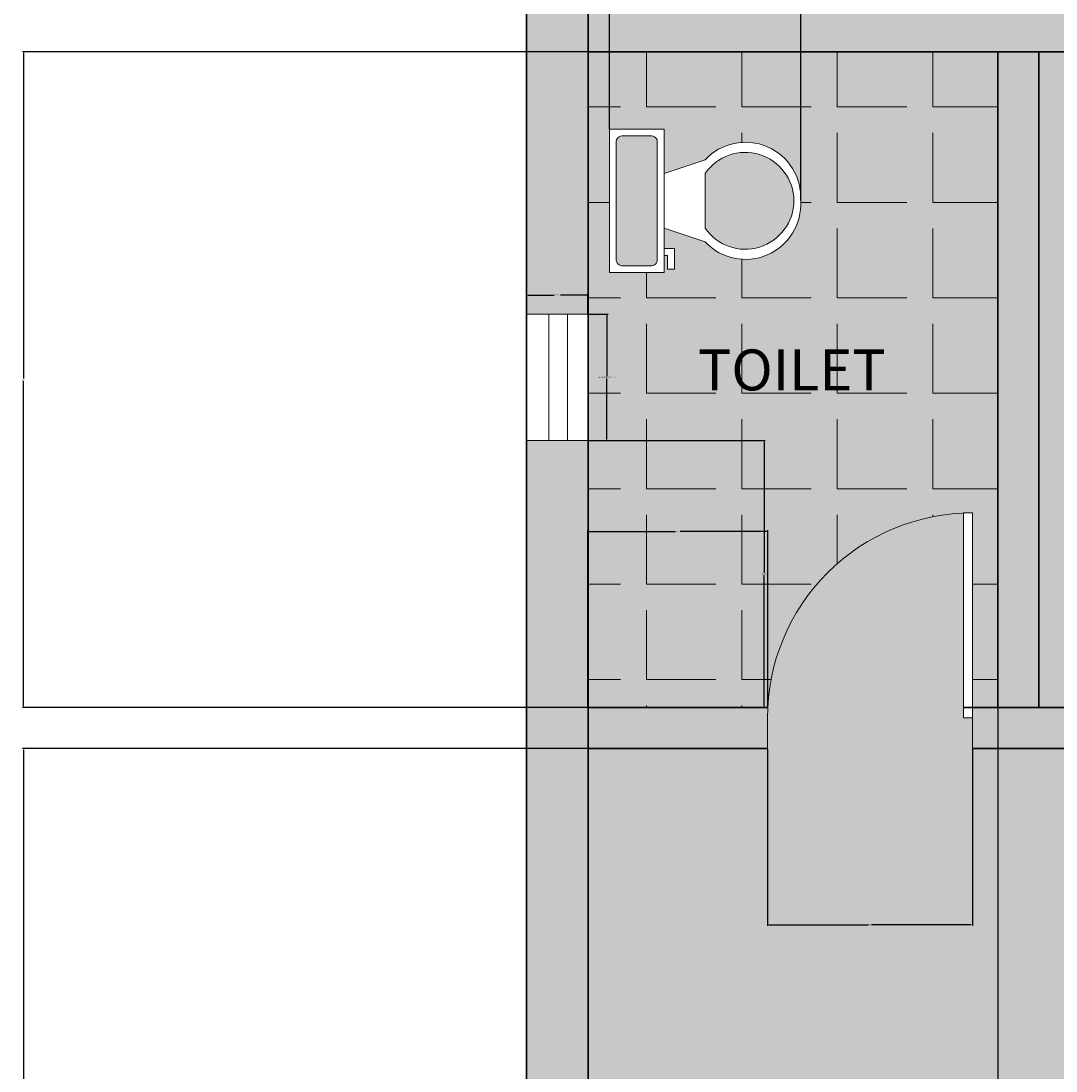
# Model space of a CAD drawing. Units: inches. Extents: x 3024 to 3952, y 1308 to 1863.
# Tile 2 of 29: x 3024 to 3175, y 1479 to 1633. Entities that reach past the tile are written whole.
import ezdxf

# ---------------------------------------------------------------- set-up
doc = ezdxf.new("R2010")
doc.units = ezdxf.units.IN
for name, color, linetype, lineweight in [('A-ANNO-DIMS', 2, 'Continuous', 18), ('A-AREA-IDEN', 7, 'Continuous', 18), ('A-DOOR', 4, 'Continuous', 18), ('A-FLOR-FIXT', 9, 'Continuous', 18), ('A-FLOR-FIXT-PATT', 7, 'Continuous', 13), ('A-FLOR-TILE-PATT', 7, 'Continuous', 13), ('A-GLAZ', 4, 'Continuous', 18), ('A-WALL', 7, 'Continuous', 35)]:
    doc.layers.add(name, color=color, linetype=linetype, lineweight=lineweight)
doc.layers.add('A-FLOR-PATT', color=254, linetype='Continuous', lineweight=13, true_color=0xfeeab9)
doc.layers.add('A-WALL-PATT', color=254, linetype='Continuous', lineweight=13, true_color=0xcecce6)
doc.styles.get("Standard").update_dxf_attribs({"font": 'arial.ttf'})
doc.dimstyles.get("Standard").update_dxf_attribs({"dimtxt": 0.18, "dimasz": 0.18, "dimexe": 0.18, "dimexo": 0.0625, "dimgap": 0.09, "dimtad": 0, "dimtih": 1, "dimtoh": 1, "dimdec": 4, "dimzin": 0, "dimdsep": 46, "dimtxsty": 'Standard', "dimcen": 0.09, "dimadec": 0, "dimazin": 0, "dimtfac": 1, "dimtdec": 4, "dimtofl": 0, "dimtmove": 0, "dimatfit": 3, "dimfxl": 1, "dimtolj": 1, "dimtzin": 0, "dimarcsym": 0})

# ---------------------------------------------------------------- blocks, each defined once
blk = doc.blocks.new('*U10')
for p, q in [((0, 0), (0, 6)), ((40, 0), (40, 6))]:
    blk.add_line(p, q)
blk.add_lwpolyline([(0, 0), (0, -40), (1.75, -40), (1.75, 0)], close=True)
blk.add_arc((0, 0), 40, 270, 0)
blk = doc.blocks.new('*U12')
for p, q in [((9.5, -6), (9.5, -2)), ((-10, -8.5), (-8, -8.5)), ((-10, -9.5), (-10, -8.5)), ((-8, -8.5), (-8, -8)), ((-7, -8), (-7, -9.5)), ((-4, -8), (-6, -14)), ((4, -8), (6, -14)), ((-7, -9.5), (-10, -9.5)), ((4, -14), (-4, -14))]:
    blk.add_line(p, q)
blk.add_lwpolyline([(10.5, -8), (10.5, 0), (-10.5, 0), (-10.5, -8)], close=True)
for points in [[(8.5, -1), (-8.5, -1)], [(-9.5, -2), (-9.5, -6)], [(-8.5, -7), (8.5, -7)]]:
    blk.add_lwpolyline(points)
for centre, radius, start, end in [((-8.625, -1.875), 0.8839, 81.8699, 188.1301), ((8.625, -1.875), 0.8839, 351.8699, 98.1301), ((-8.625, -6.125), 0.8839, 171.869898, 278.1301), ((8.625, -6.125), 0.8839, 261.8699, 8.1301), ((-0.4772, -19.9188), 8.0953, 133.01722, 273.38), ((0.0374, -19.8731), 7.127, 124.50543, 269.7), ((-0.0373, -19.8731), 7.127, 270.3, 55.4946), ((0.4773, -19.9188), 8.0953, 266.62, 46.9828)]:
    blk.add_arc(centre, radius, start, end)
blk = doc.blocks.new('WIN-BATH-18p5IN')
for p, q in [((0, 5.99), (0, 9)), ((18.52, 6.41), (18.52, 9)), ((18.52, 6.41), (18.52, 5.99)), ((0, 3.28), (0, 0)), ((18.52, 3.69), (18.52, 0))]:
    blk.add_line(p, q)
blk.add_lwpolyline([(0, 5.99), (18.52, 5.99), (18.52, 3.28), (0, 3.28)], close=True)
blk = doc.blocks.new('*D26')
at = {"layer": 'A-ANNO-DIMS', "color": 0, "lineweight": -2, "transparency": 16777216}
for p, q in [((3106.83, 1590.21), (3109.72, 1590.21)), ((3109.54, 1590.03), (3109.54, 1581.14)), ((3109.54, 1571.87), (3109.54, 1580.77)), ((3106.83, 1571.69), (3109.72, 1571.69))]:
    blk.add_line(p, q, dxfattribs=at)
at = {"layer": 'A-ANNO-DIMS', "color": 0, "transparency": 16777216}
for points in [[(3109.51, 1590.03), (3109.57, 1590.03), (3109.54, 1590.21)], [(3109.51, 1571.87), (3109.57, 1571.87), (3109.54, 1571.69)]]:
    blk.add_solid(points, dxfattribs=at)
at = {"layer": 'Defpoints', "color": 0, "transparency": 16777216}
for p in [(3106.76, 1590.21), (3106.76, 1571.69), (3109.54, 1571.69)]:
    blk.add_point(p, dxfattribs=at)
at = {"layer": 'A-ANNO-DIMS', "color": 0, "transparency": 16777216, "insert": (3109.54, 1580.95), "char_height": 0.18, "attachment_point": 5}
blk.add_mtext('\\A1;BATH WINDOW 19 TYP.', dxfattribs=at)
blk = doc.blocks.new('*D27')
at = {"layer": 'A-ANNO-DIMS', "color": 0, "lineweight": -2, "transparency": 16777216}
for p, q in [((3097.76, 1590.28), (3097.76, 1593.17)), ((3097.94, 1592.99), (3101.81, 1592.99)), ((3106.58, 1592.99), (3102.72, 1592.99)), ((3106.76, 1590.28), (3106.76, 1593.17))]:
    blk.add_line(p, q, dxfattribs=at)
at = {"layer": 'A-ANNO-DIMS', "color": 0, "transparency": 16777216}
for points in [[(3097.94, 1593.02), (3097.94, 1592.96), (3097.76, 1592.99)], [(3106.58, 1593.02), (3106.58, 1592.96), (3106.76, 1592.99)]]:
    blk.add_solid(points, dxfattribs=at)
at = {"layer": 'Defpoints', "color": 0, "transparency": 16777216}
for p in [(3106.76, 1592.99), (3097.76, 1590.21), (3106.76, 1590.21)]:
    blk.add_point(p, dxfattribs=at)
at = {"layer": 'A-ANNO-DIMS', "color": 0, "transparency": 16777216, "insert": (3102.26, 1592.99), "char_height": 0.18, "attachment_point": 5}
blk.add_mtext('\\A1;9 TYP.', dxfattribs=at)
blk = doc.blocks.new('*D43')
at = {"layer": 'A-ANNO-DIMS', "color": 0, "lineweight": -2, "transparency": 16777216}
for p, q in [((3106.7, 1628.61), (3023.95, 1628.61)), ((3024.13, 1628.43), (3024.13, 1580.79)), ((3024.13, 1532.79), (3024.13, 1580.42)), ((3106.7, 1532.61), (3023.95, 1532.61))]:
    blk.add_line(p, q, dxfattribs=at)
at = {"layer": 'A-ANNO-DIMS', "color": 0, "transparency": 16777216}
for points in [[(3024.1, 1628.43), (3024.16, 1628.43), (3024.13, 1628.61)], [(3024.1, 1532.79), (3024.16, 1532.79), (3024.13, 1532.61)]]:
    blk.add_solid(points, dxfattribs=at)
at = {"layer": 'Defpoints', "color": 0, "transparency": 16777216}
for p in [(3106.76, 1628.61), (3024.13, 1532.61), (3106.76, 1532.61)]:
    blk.add_point(p, dxfattribs=at)
at = {"layer": 'A-ANNO-DIMS', "color": 0, "transparency": 16777216, "insert": (3024.13, 1580.61), "char_height": 0.18, "attachment_point": 5}
blk.add_mtext('\\A1;96', dxfattribs=at)
blk = doc.blocks.new('*D44')
at = {"layer": 'A-ANNO-DIMS', "color": 0, "lineweight": -2, "transparency": 16777216}
for p, q in [((3106.7, 1526.61), (3023.95, 1526.61)), ((3024.13, 1526.43), (3024.13, 1441.91)), ((3024.13, 1357.03), (3024.13, 1441.54)), ((3106.7, 1356.85), (3023.95, 1356.85))]:
    blk.add_line(p, q, dxfattribs=at)
at = {"layer": 'A-ANNO-DIMS', "color": 0, "transparency": 16777216}
for points in [[(3024.1, 1526.43), (3024.16, 1526.43), (3024.13, 1526.61)], [(3024.1, 1357.03), (3024.16, 1357.03), (3024.13, 1356.85)]]:
    blk.add_solid(points, dxfattribs=at)
at = {"layer": 'Defpoints', "color": 0, "transparency": 16777216}
for p in [(3106.76, 1526.61), (3024.13, 1356.85), (3106.76, 1356.85)]:
    blk.add_point(p, dxfattribs=at)
at = {"layer": 'A-ANNO-DIMS', "color": 0, "transparency": 16777216, "insert": (3024.13, 1441.73), "char_height": 0.18, "attachment_point": 5}
blk.add_mtext('\\A1;169.76', dxfattribs=at)
blk = doc.blocks.new('*D47')
at = {"layer": 'A-ANNO-DIMS', "color": 0, "lineweight": -2, "transparency": 16777216}
for p, q in [((3106.76, 1628.54), (3106.76, 1321.89)), ((3166.76, 1628.54), (3166.76, 1321.89)), ((3106.94, 1322.07), (3136.54, 1322.07)), ((3166.58, 1322.07), (3136.98, 1322.07))]:
    blk.add_line(p, q, dxfattribs=at)
at = {"layer": 'A-ANNO-DIMS', "color": 0, "transparency": 16777216}
for points in [[(3106.94, 1322.1), (3106.94, 1322.04), (3106.76, 1322.07)], [(3166.58, 1322.1), (3166.58, 1322.04), (3166.76, 1322.07)]]:
    blk.add_solid(points, dxfattribs=at)
at = {"layer": 'Defpoints', "color": 0, "transparency": 16777216}
for p in [(3106.76, 1628.61), (3166.76, 1628.61), (3166.76, 1322.07)]:
    blk.add_point(p, dxfattribs=at)
at = {"layer": 'A-ANNO-DIMS', "color": 0, "transparency": 16777216, "insert": (3136.76, 1322.07), "char_height": 0.18, "attachment_point": 5}
blk.add_mtext('\\A1;60', dxfattribs=at)
blk = doc.blocks.new('*D53')
at = {"layer": 'A-ANNO-DIMS', "color": 0, "lineweight": -2, "transparency": 16777216}
for p, q in [((3106.76, 1532.67), (3106.76, 1558.56)), ((3133.07, 1532.67), (3133.07, 1558.56)), ((3106.94, 1558.38), (3119.59, 1558.38)), ((3132.89, 1558.38), (3120.24, 1558.38))]:
    blk.add_line(p, q, dxfattribs=at)
at = {"layer": 'A-ANNO-DIMS', "color": 0, "transparency": 16777216}
for points in [[(3106.94, 1558.41), (3106.94, 1558.35), (3106.76, 1558.38)], [(3132.89, 1558.41), (3132.89, 1558.35), (3133.07, 1558.38)]]:
    blk.add_solid(points, dxfattribs=at)
at = {"layer": 'Defpoints', "color": 0, "transparency": 16777216}
for p in [(3133.07, 1558.38), (3106.76, 1532.61), (3133.07, 1532.61)]:
    blk.add_point(p, dxfattribs=at)
at = {"layer": 'A-ANNO-DIMS', "color": 0, "transparency": 16777216, "insert": (3119.92, 1558.38), "char_height": 0.18, "attachment_point": 5}
blk.add_mtext('\\A1;26.3', dxfattribs=at)
blk = doc.blocks.new('*D54')
at = {"layer": 'A-ANNO-DIMS', "color": 0, "lineweight": -2, "transparency": 16777216}
for p, q in [((3133.03, 1526.54), (3133.03, 1500.65)), ((3163.03, 1526.54), (3163.03, 1500.65)), ((3133.21, 1500.83), (3147.81, 1500.83)), ((3162.85, 1500.83), (3148.25, 1500.83))]:
    blk.add_line(p, q, dxfattribs=at)
at = {"layer": 'A-ANNO-DIMS', "color": 0, "transparency": 16777216}
for points in [[(3133.21, 1500.86), (3133.21, 1500.8), (3133.03, 1500.83)], [(3162.85, 1500.86), (3162.85, 1500.8), (3163.03, 1500.83)]]:
    blk.add_solid(points, dxfattribs=at)
at = {"layer": 'Defpoints', "color": 0, "transparency": 16777216}
for p in [(3133.03, 1526.61), (3163.03, 1526.61), (3133.03, 1500.83)]:
    blk.add_point(p, dxfattribs=at)
at = {"layer": 'A-ANNO-DIMS', "color": 0, "transparency": 16777216, "insert": (3148.03, 1500.83), "char_height": 0.18, "attachment_point": 5}
blk.add_mtext('\\A1;30', dxfattribs=at)
blk = doc.blocks.new('*D76')
at = {"layer": 'A-ANNO-DIMS', "color": 0, "lineweight": -2, "transparency": 16777216}
for p, q in [((3106.83, 1571.69), (3132.72, 1571.69)), ((3132.54, 1571.51), (3132.54, 1552.33)), ((3132.54, 1532.79), (3132.54, 1551.97)), ((3106.83, 1532.61), (3132.72, 1532.61))]:
    blk.add_line(p, q, dxfattribs=at)
at = {"layer": 'A-ANNO-DIMS', "color": 0, "transparency": 16777216}
for points in [[(3132.51, 1571.51), (3132.57, 1571.51), (3132.54, 1571.69)], [(3132.51, 1532.79), (3132.57, 1532.79), (3132.54, 1532.61)]]:
    blk.add_solid(points, dxfattribs=at)
at = {"layer": 'Defpoints', "color": 0, "transparency": 16777216}
for p in [(3106.76, 1571.69), (3106.76, 1532.61), (3132.54, 1532.61)]:
    blk.add_point(p, dxfattribs=at)
at = {"layer": 'A-ANNO-DIMS', "color": 0, "transparency": 16777216, "insert": (3132.54, 1552.15), "char_height": 0.18, "attachment_point": 5}
blk.add_mtext('\\A1;39.086', dxfattribs=at)
blk = doc.blocks.new('*D80')
at = {"layer": 'A-ANNO-DIMS', "color": 0, "lineweight": -2, "transparency": 16777216}
for p, q in [((3109.9, 1617.34), (3109.9, 1862.78)), ((3137.9, 1606.84), (3137.9, 1862.78)), ((3110.08, 1862.6), (3123.68, 1862.6)), ((3137.72, 1862.6), (3124.12, 1862.6))]:
    blk.add_line(p, q, dxfattribs=at)
at = {"layer": 'A-ANNO-DIMS', "color": 0, "transparency": 16777216}
for points in [[(3110.08, 1862.63), (3110.08, 1862.57), (3109.9, 1862.6)], [(3137.72, 1862.63), (3137.72, 1862.57), (3137.9, 1862.6)]]:
    blk.add_solid(points, dxfattribs=at)
at = {"layer": 'Defpoints', "color": 0, "transparency": 16777216}
for p in [(3137.9, 1862.6), (3109.9, 1617.28), (3137.9, 1606.78)]:
    blk.add_point(p, dxfattribs=at)
at = {"layer": 'A-ANNO-DIMS', "color": 0, "transparency": 16777216, "insert": (3123.9, 1862.6), "char_height": 0.18, "attachment_point": 5}
blk.add_mtext('\\A1;28', dxfattribs=at)

msp = doc.modelspace()

# ---------------------------------------------------------------- hatches: boundary and pattern name
at = {"layer": 'A-FLOR-FIXT-PATT'}
h = msp.add_hatch(color=256, dxfattribs=at)
h.dxf.hatch_style = 1
h.paths.add_polyline_path([(3116.9039, 1615.2821, 0.50000012), (3115.9039, 1616.2821), (3111.9039, 1616.2821, 0.50000012), (3110.9039, 1615.2821), (3110.9039, 1598.2821, 0.50000012), (3111.9039, 1597.2821), (3115.9039, 1597.2821, 0.50000012), (3116.9039, 1598.2821)])
h.paths.add_polyline_path([(3123.9039, 1610.7822), (3123.9039, 1602.7822, 0.73453329), (3136.9039, 1606.7822, 0.73452973)])
at = {"layer": 'A-FLOR-PATT', "transparency": 33554531}
h = msp.add_hatch(color=256, dxfattribs=at)
h.dxf.hatch_style = 1
h.paths.add_polyline_path([(3166.764, 1628.6064), (3106.764, 1628.6064), (3106.764, 1532.6064), (3133.066, 1532.6064, -0.38700389), (3161.716, 1561.0777), (3161.716, 1561.1064), (3163.0285, 1561.1064), (3163.0285, 1532.6064), (3166.764, 1532.6064)])
h.paths.add_polyline_path([(3123.904, 1600.7821), (3117.9039, 1602.7821), (3117.9039, 1599.7821), (3119.4039, 1599.7821), (3119.4039, 1596.7821), (3118.4039, 1596.7821), (3118.4039, 1598.7821), (3117.9039, 1598.7821), (3117.9039, 1596.2821), (3109.9039, 1596.2821), (3109.9039, 1617.2821), (3117.9039, 1617.2821), (3117.9039, 1610.7821), (3123.9038, 1612.7821, -0.70257121), (3137.9039, 1606.7822, -0.70256205)], flags=16)
h.paths.add_polyline_path([(3123.9039, 1602.7822), (3123.9039, 1610.7822, -0.73453329), (3136.9039, 1606.7822, -0.73452973)], flags=0)
h.paths.add_polyline_path([(3116.1539, 1597.2821), (3111.9039, 1597.2821, -0.41421356), (3110.9039, 1598.0321), (3110.9039, 1615.2821, -0.41421356), (3111.6539, 1616.2821), (3115.9039, 1616.2821, -0.41421356), (3116.9039, 1615.5321), (3116.9039, 1598.2821, -0.41421356)], flags=0)
h.paths.add_polyline_path([(3292.764, 1778.6064), (3232.764, 1778.6064), (3232.764, 1694.6064), (3236.1584, 1694.6064), (3236.1584, 1723.1064), (3237.4709, 1723.1064), (3237.4709, 1723.0777, -0.38700389), (3266.1209, 1694.6064), (3292.764, 1694.6064)])
h.paths.add_polyline_path([(3263.6843, 1748.8282, -0.70256205), (3257.6842, 1762.8281), (3259.6842, 1768.8281), (3256.6842, 1768.8281), (3256.6842, 1767.3281), (3253.6842, 1767.3281), (3253.6842, 1768.3281), (3255.6842, 1768.3281), (3255.6842, 1768.8281), (3253.1842, 1768.8281), (3253.1842, 1776.8281), (3274.1842, 1776.8281), (3274.1842, 1768.8281), (3267.6842, 1768.8281), (3269.6842, 1762.8282, -0.70257121)], flags=16)
h.paths.add_polyline_path([(3263.6842, 1749.8282, -0.73452973), (3259.6842, 1762.8281), (3267.6843, 1762.8281, -0.73453329)], flags=0)
h.paths.add_polyline_path([(3255.1842, 1769.8281, -0.41421356), (3254.1842, 1770.5781), (3254.1842, 1774.8281, -0.41421356), (3254.9342, 1775.8281), (3272.1842, 1775.8281, -0.41421356), (3273.1842, 1775.0781), (3273.1842, 1770.8281, -0.41421356), (3272.4342, 1769.8281)], flags=0)
h.paths.add_polyline_path([(3460.764, 1778.6064), (3412.764, 1778.6064), (3412.764, 1745.5689, -0.38700389), (3441.2353, 1716.9189), (3441.264, 1716.9189), (3441.264, 1715.6064), (3412.764, 1715.6064), (3412.764, 1694.6064), (3460.764, 1694.6064)])
h.paths.add_polyline_path([(3121.3033, 1577.378), (3153.693, 1577.378), (3153.693, 1586.6752), (3121.3033, 1586.6752)], flags=24)
h.paths.add_polyline_path([(3245.8895, 1726.2997), (3278.2793, 1726.2997), (3278.2793, 1735.5968), (3245.8895, 1735.5968)], flags=24)
h.paths.add_polyline_path([(3419.204, 1753.8578), (3453.3997, 1753.8578), (3453.3997, 1762.9956), (3419.204, 1762.9956)], flags=24)
at = {"layer": 'A-FLOR-PATT', "transparency": 33554528}
h = msp.add_hatch(color=256, dxfattribs=at)
h.dxf.hatch_style = 1
h.paths.add_polyline_path([(3460.764, 1688.6064), (3412.764, 1688.6064), (3412.764, 1694.6064), (3460.764, 1694.6064), (3460.764, 1778.6064), (3406.764, 1778.6064), (3406.764, 1759.9514), (3318.2981, 1759.9514), (3318.2981, 1658.6064), (3322.5356, 1658.6064), (3322.5356, 1652.6064), (3292.764, 1652.6064), (3292.764, 1778.6064), (3106.764, 1778.6064), (3106.764, 1628.6064), (3172.764, 1628.6064), (3172.764, 1532.6064), (3166.764, 1532.6064), (3166.764, 1628.6064), (3106.764, 1628.6064), (3106.764, 1356.8452), (3202.812, 1356.8452), (3202.812, 1354.2534), (3202.812, 1353.8388), (3202.812, 1351.1212), (3202.812, 1347.8452), (3277.764, 1347.8452), (3277.764, 1353.8452), (3277.764, 1356.8452), (3277.764, 1442.6064), (3460.764, 1442.6064)])
h.paths.add_polyline_path([(3216.238, 1527.2064), (3216.238, 1491.2064), (3214.663, 1491.2064), (3214.663, 1491.2409, -0.39662236), (3180.243, 1526.6064), (3163.0285, 1526.6064), (3163.0285, 1531.1064), (3161.716, 1531.1064), (3161.716, 1561.1064), (3163.0285, 1561.1064), (3163.0285, 1531.1064), (3163.0285, 1526.6064), (3180.243, 1526.6064, 0.39662236), (3214.663, 1491.2409), (3214.663, 1527.2064)], flags=16)
h.paths.add_polyline_path([(3227.364, 1649.8972), (3191.364, 1649.8972), (3191.364, 1651.4722), (3227.364, 1651.4722)], flags=16)
h.paths.add_polyline_path([(3323.1172, 1606.7362), (3323.8545, 1606.8514), (3323.8545, 1594.8241), (3323.1172, 1594.9393)], flags=16)
h.paths.add_polyline_path([(3324.2232, 1606.909), (3330.1216, 1607.8307), (3330.1216, 1614.1093), (3339.3495, 1614.1093), (3340.2711, 1620.0078), (3352.4136, 1620.0078), (3353.3353, 1614.1093), (3359.9941, 1614.1093), (3360.9157, 1620.0078), (3373.0582, 1620.0078), (3373.9799, 1614.1093), (3383.2077, 1614.1093), (3383.2077, 1607.8307), (3389.1062, 1606.909), (3389.1062, 1594.7665), (3383.2077, 1593.8449), (3383.2077, 1587.5663), (3373.9799, 1587.5663), (3373.0583, 1581.6678), (3360.9157, 1581.6678), (3359.9941, 1587.5663), (3353.3353, 1587.5663), (3352.4136, 1581.6678), (3340.2711, 1581.6678), (3339.3495, 1587.5663), (3330.1216, 1587.5663), (3330.1216, 1593.8449), (3324.2232, 1594.7665)], flags=16)
h.paths.add_polyline_path([(3236.1584, 1693.1064), (3236.1584, 1723.1064), (3237.4709, 1723.1064), (3237.4709, 1693.1064)], flags=16)
h.paths.add_polyline_path([(3373.2158, 1600.6847), (3373.7965, 1600.7303), (3374.3268, 1600.7874), (3374.8132, 1600.8531), (3375.2621, 1600.9247), (3375.6801, 1600.9991), (3376.0736, 1601.0735), (3376.6855, 1601.19), (3377.366, 1601.3023), (3378.0667, 1601.3814), (3378.8026, 1601.4123), (3379.5865, 1601.3839), (3380.4537, 1601.2948), (3381.301, 1601.1717), (3382.0317, 1601.0433), (3382.4398, 1600.9607), (3382.6252, 1600.9201), (3382.919, 1600.8507), (3382.9044, 1600.8531), (3382.842, 1600.8678), (3382.7541, 1600.8896), (3382.6252, 1600.9201), (3382.4398, 1600.9607), (3382.1868, 1601.0119), (3381.8738, 1601.0711), (3381.5125, 1601.1346), (3381.1149, 1601.1988), (3380.6928, 1601.2601), (3380.2581, 1601.3149), (3379.8226, 1601.3597), (3379.3984, 1601.3908), (3378.9944, 1601.4054), (3378.6092, 1601.4042), (3378.2384, 1601.3886), (3377.8777, 1601.36), (3377.5227, 1601.32), (3377.1691, 1601.2698), (3376.8127, 1601.211), (3376.4491, 1601.145), (3376.0736, 1601.0735), (3375.4177, 1600.9494), (3374.5542, 1600.8119), (3373.5044, 1600.6988)], flags=0)
h.paths.add_polyline_path([(3380.0253, 1596.7351), (3380.499, 1596.6659), (3380.9706, 1596.6119), (3381.4375, 1596.5791), (3381.8971, 1596.5736), (3382.5886, 1596.6167), (3382.7848, 1596.6692), (3382.1465, 1596.5706), (3381.236, 1596.5815), (3380.3199, 1596.6865)], flags=0)
h.paths.add_polyline_path([(3369.6414, 1603.9617), (3370.1589, 1604.0021), (3370.6218, 1604.0539), (3371.0335, 1604.1173), (3371.3978, 1604.1921), (3371.7181, 1604.2785), (3371.9984, 1604.3761), (3372.2441, 1604.483), (3372.4611, 1604.5972), (3372.655, 1604.7163), (3372.8317, 1604.8384), (3372.9968, 1604.9611), (3373.3703, 1605.2455), (3373.8426, 1605.5328), (3374.4624, 1605.7539), (3375.1058, 1605.8302), (3375.7221, 1605.8261), (3376.4109, 1605.76), (3377.1534, 1605.6376), (3377.8945, 1605.473), (3378.1382, 1605.409), (3377.7394, 1605.5074), (3377.3509, 1605.5937), (3376.9704, 1605.6677), (3376.5999, 1605.7288), (3376.2417, 1605.7762), (3375.8979, 1605.8092), (3375.5707, 1605.8271), (3375.2621, 1605.8291), (3374.9745, 1605.8146), (3374.7092, 1605.7832), (3374.4647, 1605.7359), (3374.239, 1605.6742), (3374.0298, 1605.5996), (3373.835, 1605.5134), (3373.6525, 1605.4171), (3373.4801, 1605.3123), (3373.3156, 1605.2002), (3373.1562, 1605.0825), (3372.7603, 1604.781), (3372.236, 1604.4588), (3371.5738, 1604.2283), (3370.8493, 1604.0794), (3369.9262, 1603.976)], flags=0)
h.paths.add_polyline_path([(3366.7533, 1606.5832), (3367.1713, 1606.5519), (3367.5378, 1606.5374), (3367.8568, 1606.5394), (3368.1325, 1606.5573), (3368.3694, 1606.5903), (3368.5717, 1606.6377), (3368.7438, 1606.6988), (3368.89, 1606.7728), (3369.0146, 1606.8591), (3369.121, 1606.9568), (3369.2094, 1607.0646), (3369.2792, 1607.181), (3369.3295, 1607.3046), (3369.3596, 1607.4339), (3369.3688, 1607.5676), (3369.3565, 1607.7042), (3369.3218, 1607.8422), (3369.2649, 1607.9804), (3369.1893, 1608.1187), (3369.0993, 1608.2569), (3368.9992, 1608.3952), (3368.8934, 1608.5334), (3368.7861, 1608.6717), (3368.6817, 1608.8099), (3368.4212, 1609.1804), (3368.2685, 1609.7106), (3368.4883, 1610.1814), (3369.0537, 1610.4604), (3369.6717, 1610.5097), (3370.2812, 1610.3612), (3370.4805, 1610.2968), (3370.1882, 1610.3839), (3369.9284, 1610.4472), (3369.6905, 1610.4842), (3369.4662, 1610.4933), (3369.2555, 1610.4765), (3369.0608, 1610.4367), (3368.884, 1610.3767), (3368.7274, 1610.2994), (3368.5931, 1610.2077), (3368.4833, 1610.1045), (3368.4002, 1609.9927), (3368.3451, 1609.8747), (3368.3166, 1609.7517), (3368.3127, 1609.6244), (3368.331, 1609.4935), (3368.3696, 1609.3597), (3368.4261, 1609.2237), (3368.4985, 1609.0863), (3368.5845, 1608.9482), (3368.6817, 1608.8099), (3368.7861, 1608.6717), (3368.8934, 1608.5334), (3368.9992, 1608.3952), (3369.0993, 1608.2569), (3369.3398, 1607.8876), (3369.3941, 1607.2896), (3368.9774, 1606.7817), (3368.3928, 1606.5742), (3367.7162, 1606.5303), (3367.0044, 1606.5585)], flags=0)
h.paths.add_polyline_path([(3362.1859, 1610.2589), (3362.5478, 1610.2845), (3362.8348, 1610.3275), (3363.0585, 1610.3863), (3363.2303, 1610.4595), (3363.3619, 1610.5457), (3363.463, 1610.6432), (3363.5376, 1610.7502), (3363.5876, 1610.8643), (3363.6153, 1610.9834), (3363.6229, 1611.1055), (3363.6125, 1611.2283), (3363.5861, 1611.3496), (3363.5462, 1611.4673), (3363.4949, 1611.5797), (3363.4358, 1611.6871), (3363.3723, 1611.7902), (3363.3081, 1611.8897), (3363.2468, 1611.9863), (3363.192, 1612.0808), (3363.0258, 1612.4261), (3363.3371, 1612.8672), (3363.9008, 1612.9782), (3364.4822, 1612.9641), (3365.1098, 1612.9074), (3365.328, 1612.8805), (3364.9615, 1612.9208), (3364.6426, 1612.9496), (3364.3668, 1612.9669), (3364.1299, 1612.9726), (3363.9276, 1612.9669), (3363.7555, 1612.9496), (3363.6093, 1612.9208), (3363.4848, 1612.8805), (3363.3782, 1612.8289), (3363.2889, 1612.7672), (3363.2169, 1612.6969), (3363.1622, 1612.6193), (3363.1247, 1612.5361), (3363.1046, 1612.4484), (3363.1017, 1612.358), (3363.1161, 1612.266), (3363.1472, 1612.1738), (3363.192, 1612.0808), (3363.2468, 1611.9863), (3363.3081, 1611.8897), (3363.3723, 1611.7902), (3363.4358, 1611.6871), (3363.6363, 1611.323), (3363.5979, 1610.7003), (3363.0863, 1610.3651), (3362.3983, 1610.2622)], flags=0)
h.paths.add_polyline_path([(3352.356, 1581.2991), (3352.2408, 1580.5618), (3340.4439, 1580.5618), (3340.3287, 1581.2991)], flags=16)
h.paths.add_polyline_path([(3340.4439, 1621.1137), (3352.2408, 1621.1137), (3352.356, 1620.3764), (3340.3287, 1620.3764)], flags=16)
h.paths.add_polyline_path([(3278.4282, 1504.7424), (3290.3831, 1504.7424), (3290.3831, 1502.7499), (3291.0473, 1502.7499), (3291.0473, 1494.7799), (3290.3831, 1494.7799), (3290.3831, 1494.1158), (3291.0473, 1494.1158), (3291.0473, 1486.1458), (3290.3831, 1486.1458), (3290.3831, 1484.1533), (3291.0473, 1484.1533), (3291.0473, 1483.4892, -0.09090909), (3291.0473, 1468.8776), (3291.0473, 1468.2135), (3290.3831, 1468.2135), (3290.3831, 1464.8926), (3278.4282, 1464.8926), (3278.4282, 1472.8626), (3277.764, 1473.5268), (3277.764, 1478.84), (3278.4282, 1479.5042)], flags=16)
h.paths.add_polyline_path([(3278.7603, 1504.4103), (3290.051, 1504.4103), (3290.051, 1465.2247), (3278.7603, 1465.2247)], flags=0)
h.paths.add_polyline_path([(3123.904, 1600.7821), (3117.9039, 1602.7821), (3117.9039, 1599.7821), (3119.4039, 1599.7821), (3119.4039, 1596.7821), (3118.4039, 1596.7821), (3118.4039, 1598.7821), (3117.9039, 1598.7821), (3117.9039, 1596.2821), (3109.9039, 1596.2821), (3109.9039, 1617.2821), (3117.9039, 1617.2821), (3117.9039, 1610.7821), (3123.9038, 1612.7821, -0.70257121), (3137.9039, 1606.7822, -0.70256205)], flags=16)
h.paths.add_polyline_path([(3123.9039, 1602.7822), (3123.9039, 1610.7822, -0.73453329), (3136.9039, 1606.7822, -0.73452973)], flags=0)
h.paths.add_polyline_path([(3177.972, 1689.6473), (3109.2405, 1689.6473), (3109.2405, 1741.1959), (3177.972, 1741.1959)], flags=16)
h.paths.add_polyline_path([(3373.0006, 1581.2991), (3372.8854, 1580.5618), (3361.0885, 1580.5618), (3360.9733, 1581.2991)], flags=16)
h.paths.add_polyline_path([(3361.0885, 1621.1137), (3372.8854, 1621.1137), (3373.0006, 1620.3764), (3360.9733, 1620.3764)], flags=16)
h.paths.add_polyline_path([(3116.9039, 1598.2821, -0.41421356), (3116.1539, 1597.2821), (3111.9039, 1597.2821, -0.41421356), (3110.9039, 1598.0321), (3110.9039, 1615.2821, -0.41421356), (3111.6539, 1616.2821), (3115.9039, 1616.2821, -0.41421356), (3116.9039, 1615.5321)], flags=0)
h.paths.add_polyline_path([(3121.6122, 1728.1369), (3121.6122, 1696.5205), (3110.2715, 1696.5205), (3110.2715, 1714.3906), (3121.6122, 1714.3906), (3121.6122, 1716.4526), (3110.2715, 1716.4526), (3110.2715, 1734.3228), (3123.3304, 1734.3228), (3123.3304, 1729.8552), (3134.6711, 1741.1959), (3134.6711, 1728.1369)], flags=0)
h.paths.add_polyline_path([(3389.4748, 1606.8514), (3390.2122, 1606.7362), (3390.2122, 1594.9393), (3389.4748, 1594.8241)], flags=16)
h.paths.add_polyline_path([(3257.6842, 1762.8281), (3259.6842, 1768.8281), (3256.6842, 1768.8281), (3256.6842, 1767.3281), (3253.6842, 1767.3281), (3253.6842, 1768.3281), (3255.6842, 1768.3281), (3255.6842, 1768.8281), (3253.1842, 1768.8281), (3253.1842, 1776.8281), (3274.1842, 1776.8281), (3274.1842, 1768.8281), (3267.6842, 1768.8281), (3269.6842, 1762.8282, -0.70257121), (3263.6843, 1748.8282, -0.70256205)], flags=16)
h.paths.add_polyline_path([(3259.6842, 1762.8281), (3267.6843, 1762.8281, -0.73453329), (3263.6842, 1749.8282, -0.73452973)], flags=0)
h.paths.add_polyline_path([(3411.264, 1715.6064), (3411.264, 1716.9189), (3441.264, 1716.9189), (3441.264, 1715.6064)], flags=16)
h.paths.add_polyline_path([(3178.3806, 1449.1876), (3178.3806, 1397.639), (3109.6491, 1397.639), (3109.6491, 1449.1876)], flags=16)
h.paths.add_polyline_path([(3397.1501, 1541.7146), (3419.6183, 1541.7146), (3419.6183, 1496.7783), (3397.1501, 1496.7783)], flags=16)
h.paths.add_polyline_path([(3254.1842, 1770.5781), (3254.1842, 1774.8281, -0.41421356), (3254.9342, 1775.8281), (3272.1842, 1775.8281, -0.41421356), (3273.1842, 1775.0781), (3273.1842, 1770.8281, -0.41421356), (3272.4342, 1769.8281), (3255.1842, 1769.8281, -0.41421356)], flags=0)
h.paths.add_polyline_path([(3403.672, 1500.7601), (3403.6016, 1500.3997), (3403.5328, 1500.0441), (3403.4662, 1499.6867), (3403.4027, 1499.3226), (3403.3464, 1498.9532), (3403.3025, 1498.5811), (3403.2759, 1498.2091), (3403.2714, 1497.8401), (3403.3064, 1497.2813), (3403.3491, 1497.1219), (3403.2689, 1497.6395), (3403.2778, 1498.3719), (3403.3635, 1499.0984), (3403.4889, 1499.8168), (3403.6016, 1500.3997), (3403.672, 1500.7601), (3403.744, 1501.1315), (3403.817, 1501.5205), (3403.891, 1501.9336), (3403.9656, 1502.3769), (3404.0404, 1502.8572), (3404.115, 1503.3786), (3404.2264, 1504.2311), (3404.2571, 1504.5223), (3404.1552, 1503.6598), (3404.0063, 1502.6193), (3403.8604, 1501.7518), (3403.744, 1501.1315)], flags=0)
h.paths.add_polyline_path([(3406.5868, 1505.0416), (3406.6121, 1504.5236), (3406.6492, 1504.0526), (3406.6956, 1503.624), (3406.7491, 1503.2333), (3406.8072, 1502.8759), (3406.8676, 1502.5473), (3406.9281, 1502.243), (3407.0268, 1501.7597), (3407.1416, 1501.1368), (3407.2087, 1500.3904), (3407.1804, 1499.6703), (3407.1078, 1498.9956), (3407.0074, 1498.3199), (3406.8809, 1497.6059), (3406.7403, 1496.9627), (3406.7418, 1496.9824), (3406.7491, 1497.0249), (3406.8229, 1497.3409), (3406.8364, 1497.4025), (3406.878, 1497.6078), (3406.9261, 1497.8614), (3406.9777, 1498.1526), (3407.0298, 1498.4712), (3407.0797, 1498.8068), (3407.1243, 1499.149), (3407.1607, 1499.4874), (3407.1859, 1499.8115), (3407.1978, 1500.1137), (3407.1969, 1500.3962), (3407.1841, 1500.6642), (3407.1609, 1500.9225), (3407.1284, 1501.1761), (3407.0876, 1501.43), (3407.0398, 1501.6891), (3406.9862, 1501.9585), (3406.8832, 1502.4628), (3406.7712, 1503.0713), (3406.6657, 1503.8424), (3406.5924, 1504.7735)], flags=0)
h.paths.add_polyline_path([(3409.2517, 1507.8962), (3409.2752, 1507.4282), (3409.3079, 1507.0076), (3409.3501, 1506.6314), (3409.4015, 1506.2969), (3409.4624, 1506.0009), (3409.5326, 1505.7406), (3409.6119, 1505.5128), (3409.6988, 1505.3131), (3409.7915, 1505.1368), (3409.8883, 1504.9792), (3409.9875, 1504.8356), (3410.0872, 1504.7015), (3410.1859, 1504.572), (3410.4508, 1504.2132), (3410.7205, 1503.6035), (3410.8059, 1502.8824), (3410.7619, 1502.0875), (3410.6122, 1501.2299), (3410.4402, 1500.6169), (3410.2538, 1500.0031), (3410.0536, 1499.3219), (3409.9909, 1499.0812), (3410.1761, 1499.7472), (3410.3596, 1500.3513), (3410.4512, 1500.6561), (3410.5312, 1500.9412), (3410.6013, 1501.226), (3410.6614, 1501.512), (3410.7111, 1501.7964), (3410.7496, 1502.0763), (3410.7764, 1502.3489), (3410.7909, 1502.6114), (3410.7926, 1502.8608), (3410.7808, 1503.0944), (3410.7553, 1503.31), (3410.7169, 1503.5087), (3410.6667, 1503.6921), (3410.6061, 1503.8621), (3410.5361, 1504.0203), (3410.4578, 1504.1686), (3410.3726, 1504.3088), (3410.2815, 1504.4424), (3410.1859, 1504.572), (3410.0872, 1504.7015), (3409.859, 1505.0083), (3409.5943, 1505.5117), (3409.4266, 1506.1336), (3409.324, 1506.8011), (3409.2586, 1507.6407)], flags=0)
h.paths.add_polyline_path([(3411.4914, 1510.5878), (3411.4432, 1510.1586), (3411.4054, 1509.775), (3411.38, 1509.4354), (3411.3681, 1509.1376), (3411.3698, 1508.8784), (3411.3843, 1508.6542), (3411.4112, 1508.4618), (3411.4497, 1508.2974), (3411.4994, 1508.1575), (3411.5595, 1508.0388), (3411.6296, 1507.9375), (3411.7097, 1507.851), (3411.802, 1507.7792), (3411.9096, 1507.7225), (3412.0353, 1507.6817), (3412.1821, 1507.6572), (3412.3528, 1507.6496), (3412.5505, 1507.6597), (3412.778, 1507.6879), (3413.0364, 1507.7341), (3413.3194, 1507.7955), (3413.6188, 1507.8687), (3413.9264, 1507.95), (3414.234, 1508.036), (3414.5333, 1508.1232), (3414.8163, 1508.208), (3415.0747, 1508.287), (3415.3023, 1508.3569), (3415.5007, 1508.4158), (3415.6733, 1508.4617), (3416.1158, 1508.5538), (3416.512, 1508.2591), (3416.716, 1507.6581), (3416.61, 1507.0003), (3416.3052, 1506.3411), (3415.8928, 1505.618), (3415.7339, 1505.3633), (3415.9914, 1505.791), (3416.201, 1506.1583), (3416.3666, 1506.4739), (3416.4925, 1506.7462), (3416.5828, 1506.9838), (3416.6413, 1507.1949), (3416.6725, 1507.3883), (3416.6799, 1507.5705), (3416.6662, 1507.7417), (3416.6339, 1507.9), (3416.5851, 1508.0436), (3416.5223, 1508.1709), (3416.4478, 1508.28), (3416.3639, 1508.3692), (3416.273, 1508.4368), (3416.1765, 1508.4815), (3416.0718, 1508.5047), (3415.9553, 1508.5079), (3415.8237, 1508.493), (3415.6733, 1508.4617), (3415.5007, 1508.4158), (3415.3327, 1508.3659), (3414.6495, 1508.157), (3414.0606, 1507.9855), (3413.4456, 1507.8229), (3412.8838, 1507.701), (3412.5505, 1507.6597), (3412.0748, 1507.6354), (3411.595, 1507.8883), (3411.398, 1508.4429), (3411.3624, 1508.9927), (3411.3854, 1509.5711), (3411.4578, 1510.3071)], flags=0)
h.paths.add_polyline_path([(3135.0797, 1449.1876), (3135.0797, 1436.1286), (3122.0208, 1436.1286), (3122.0208, 1404.5122), (3110.6801, 1404.5122), (3110.6801, 1422.3823), (3122.0208, 1422.3823), (3122.0208, 1424.4443), (3110.6801, 1424.4443), (3110.6801, 1442.3145), (3123.739, 1442.3145), (3123.739, 1437.8469)], flags=0)
h.paths.add_polyline_path([(3416.4944, 1514.2949), (3416.4837, 1513.8511), (3416.4893, 1513.4867), (3416.5102, 1513.1926), (3416.5451, 1512.9593), (3416.5929, 1512.7775), (3416.6524, 1512.6379), (3416.7224, 1512.531), (3416.8017, 1512.4488), (3416.8886, 1512.3882), (3416.9813, 1512.3476), (3417.0781, 1512.3251), (3417.1773, 1512.3189), (3417.277, 1512.3274), (3417.3757, 1512.3488), (3417.4713, 1512.3813), (3417.5627, 1512.4229), (3417.65, 1512.471), (3417.7338, 1512.5225), (3417.8146, 1512.5747), (3417.8931, 1512.6245), (3417.9699, 1512.6691), (3418.2968, 1512.8265), (3418.6505, 1512.4645), (3418.7037, 1511.9342), (3418.6693, 1511.3839), (3418.6076, 1510.8228), (3418.5777, 1510.5927), (3418.6197, 1510.9333), (3418.6525, 1511.2311), (3418.6759, 1511.4903), (3418.6899, 1511.7144), (3418.6946, 1511.9069), (3418.6899, 1512.0713), (3418.6759, 1512.2112), (3418.6525, 1512.33), (3418.6197, 1512.4311), (3418.5778, 1512.5177), (3418.5276, 1512.5903), (3418.4705, 1512.6488), (3418.4075, 1512.6933), (3418.3399, 1512.7237), (3418.2686, 1512.7401), (3418.1951, 1512.7424), (3418.1204, 1512.7307), (3418.0455, 1512.7055), (3417.9792, 1512.6736), (3417.65, 1512.471), (3417.5627, 1512.4229), (3417.4713, 1512.3813), (3417.3757, 1512.3488), (3417.277, 1512.3274), (3416.878, 1512.2936), (3416.5757, 1512.7549), (3416.492, 1513.3145), (3416.4808, 1514.0384)], flags=0)
h.paths.add_polyline_path([(3392.8223, 1481.9454), (3396.7707, 1481.9454), (3396.7707, 1480.9201), (3428.3585, 1480.9201), (3428.3585, 1481.9454), (3432.3069, 1481.9454), (3432.3069, 1464.8354, -0.26666697), (3392.8223, 1464.8354)], flags=16)
h.paths.add_polyline_path([(3431.203, 1547.5428), (3450.8613, 1547.5428, -0.19047621), (3450.8614, 1484.031), (3431.203, 1484.031), (3431.203, 1488.5675), (3432.3809, 1488.5675), (3432.3809, 1543.0062), (3431.203, 1543.0062)], flags=16)
h.paths.add_polyline_path([(3451.9233, 1524.86, -0.04962821), (3451.9233, 1506.7138), (3446.7921, 1506.7138), (3446.7921, 1524.86)], flags=0)
h.paths.add_polyline_path([(3460.764, 1436.6064), (3277.764, 1436.6064), (3277.764, 1356.8452), (3277.764, 1353.8452), (3460.764, 1353.8452)], flags=17)
h.paths.add_polyline_path([(3121.3033, 1577.378), (3153.693, 1577.378), (3153.693, 1586.6752), (3121.3033, 1586.6752)], flags=24)
h.paths.add_polyline_path([(3164.1457, 1464.1276), (3210.4801, 1464.1276), (3210.4801, 1473.4247), (3164.1457, 1473.4247)], flags=24)
h.paths.add_polyline_path([(3343.1909, 1505.8863), (3373.7236, 1505.8863), (3373.7236, 1515.1773), (3343.1909, 1515.1773)], flags=24)
h.paths.add_polyline_path([(3337.6353, 1564.2926), (3370.0189, 1564.2926), (3370.0189, 1573.5836), (3337.6353, 1573.5836)], flags=24)
h.paths.add_polyline_path([(3419.204, 1753.8578), (3453.3997, 1753.8578), (3453.3997, 1762.9956), (3419.204, 1762.9956)], flags=24)
h.paths.add_polyline_path([(3341.2523, 1701.0246), (3381.0761, 1701.0246), (3381.0761, 1710.3156), (3341.2523, 1710.3156)], flags=24)
h.paths.add_polyline_path([(3245.8895, 1726.2997), (3278.2793, 1726.2997), (3278.2793, 1735.5968), (3245.8895, 1735.5968)], flags=24)
h.paths.add_polyline_path([(3128.8045, 1668.6736), (3175.1389, 1668.6736), (3175.1389, 1677.9707), (3128.8045, 1677.9707)], flags=24)
h.paths.add_polyline_path([(3345.9997, 1396.0062), (3389.09, 1396.0062), (3389.09, 1405.3033), (3345.9997, 1405.3033)], flags=24)
at = {"layer": 'A-FLOR-TILE-PATT', "transparency": 33554569}
h = msp.add_hatch(dxfattribs=at)
h.set_pattern_fill('ANGLE', color=256, scale=2)
h.set_pattern_definition([(0, (0, 0), (0, 13.97), [10.16, -3.81]), (90, (0, 0), (-13.97, 9e-16), [10.16, -3.81])])
h.paths.add_polyline_path([(3292.764, 1778.6064), (3232.764, 1778.6064), (3232.764, 1694.6064), (3236.1584, 1694.6064), (3236.1584, 1723.1064), (3237.4709, 1723.1064), (3237.4709, 1723.0777, -0.38700389), (3266.1209, 1694.6064), (3292.764, 1694.6064)])
h.paths.add_polyline_path([(3263.6843, 1748.8282, -0.70256205), (3257.6842, 1762.8281), (3259.6842, 1768.8281), (3256.6842, 1768.8281), (3256.6842, 1767.3281), (3253.6842, 1767.3281), (3253.6842, 1768.3281), (3255.6842, 1768.3281), (3255.6842, 1768.8281), (3253.1842, 1768.8281), (3253.1842, 1776.8281), (3274.1842, 1776.8281), (3274.1842, 1768.8281), (3267.6842, 1768.8281), (3269.6842, 1762.8282, -0.70257121)], flags=16)
h.paths.add_polyline_path([(3263.6842, 1749.8282, -0.73452973), (3259.6842, 1762.8281), (3267.6843, 1762.8281, -0.73453329)], flags=0)
h.paths.add_polyline_path([(3255.1842, 1769.8281, -0.41421356), (3254.1842, 1770.5781), (3254.1842, 1774.8281, -0.41421356), (3254.9342, 1775.8281), (3272.1842, 1775.8281, -0.41421356), (3273.1842, 1775.0781), (3273.1842, 1770.8281, -0.41421356), (3272.4342, 1769.8281)], flags=0)
h.paths.add_polyline_path([(3460.764, 1436.6064), (3277.764, 1436.6064), (3277.764, 1356.8452), (3277.764, 1353.8452), (3460.764, 1353.8452)])
h.paths.add_polyline_path([(3166.764, 1628.6064), (3106.764, 1628.6064), (3106.764, 1532.6064), (3133.066, 1532.6064, -0.38700389), (3161.716, 1561.0777), (3161.716, 1561.1064), (3163.0285, 1561.1064), (3163.0285, 1532.6064), (3166.764, 1532.6064)])
h.paths.add_polyline_path([(3123.904, 1600.7821), (3117.9039, 1602.7821), (3117.9039, 1599.7821), (3119.4039, 1599.7821), (3119.4039, 1596.7821), (3118.4039, 1596.7821), (3118.4039, 1598.7821), (3117.9039, 1598.7821), (3117.9039, 1596.2821), (3109.9039, 1596.2821), (3109.9039, 1617.2821), (3117.9039, 1617.2821), (3117.9039, 1610.7821), (3123.9038, 1612.7821, -0.70257121), (3137.9039, 1606.7822, -0.70256205)], flags=16)
h.paths.add_polyline_path([(3123.9039, 1602.7822), (3123.9039, 1610.7822, -0.73453329), (3136.9039, 1606.7822, -0.73452973)], flags=0)
h.paths.add_polyline_path([(3116.1539, 1597.2821), (3111.9039, 1597.2821, -0.41421356), (3110.9039, 1598.0321), (3110.9039, 1615.2821, -0.41421356), (3111.6539, 1616.2821), (3115.9039, 1616.2821, -0.41421356), (3116.9039, 1615.5321), (3116.9039, 1598.2821, -0.41421356)], flags=0)
h.paths.add_polyline_path([(3245.8895, 1726.2997), (3278.2793, 1726.2997), (3278.2793, 1735.5968), (3245.8895, 1735.5968)], flags=24)
h.paths.add_polyline_path([(3345.9997, 1396.0062), (3389.09, 1396.0062), (3389.09, 1405.3033), (3345.9997, 1405.3033)], flags=24)
h.paths.add_polyline_path([(3121.3033, 1577.378), (3153.693, 1577.378), (3153.693, 1586.6752), (3121.3033, 1586.6752)], flags=24)
at = {"layer": 'A-WALL-PATT'}
h = msp.add_hatch(color=256, dxfattribs=at)
h.dxf.hatch_style = 1
h.paths.add_polyline_path([(3106.764, 1778.6064), (3140.5977, 1778.6064), (3140.5977, 1781.8824), (3140.5977, 1784.6), (3140.5977, 1787.6064), (3097.764, 1787.6064), (3097.764, 1590.213), (3101.04, 1590.213), (3103.7576, 1590.213), (3106.764, 1590.213)])
h.paths.add_polyline_path([(3253.5314, 1781.8824), (3253.5314, 1784.6), (3253.5314, 1787.6064), (3194.6826, 1787.6064), (3194.6826, 1785.0146), (3194.6826, 1784.6), (3194.6826, 1781.8824), (3194.6826, 1778.6064), (3253.5314, 1778.6064)])
h.paths.add_polyline_path([(3333.856, 1782.2838), (3333.856, 1784.7474), (3333.856, 1787.6064), (3272.0523, 1787.6064), (3272.0523, 1785.0146), (3272.0523, 1784.6), (3272.0523, 1781.8824), (3272.0523, 1778.6064), (3333.856, 1778.6064)])
h.paths.add_polyline_path([(3428.8344, 1784.6), (3428.8344, 1787.6064), (3378.3947, 1787.6064), (3378.3947, 1784.7474), (3378.3947, 1782.2838), (3378.3947, 1778.6064), (3428.8344, 1778.6064), (3428.8344, 1781.8824)], flags=17)
h.paths.add_polyline_path([(3469.764, 1787.6064), (3451.9386, 1787.6064), (3451.9386, 1785.0146), (3451.9386, 1784.6), (3451.9386, 1781.8824), (3451.9386, 1778.6064), (3460.764, 1778.6064), (3460.764, 1353.8452), (3277.764, 1353.8452), (3277.764, 1347.8452), (3469.764, 1347.8452), (3469.764, 1353.8452)])
h.paths.add_polyline_path([(3106.764, 1571.6922), (3104.1722, 1571.6922), (3103.7576, 1571.6922), (3101.04, 1571.6922), (3097.764, 1571.6922), (3097.764, 1347.8452), (3148.7271, 1347.8452), (3148.7271, 1351.1212), (3148.7271, 1353.8388), (3148.7271, 1356.8452), (3106.764, 1356.8452)])
h.paths.add_polyline_path([(3277.764, 1532.6064), (3262.7605, 1532.6064), (3262.7605, 1582.9359), (3256.7605, 1582.9359), (3256.7605, 1532.6064), (3244.2116, 1532.6064), (3216.238, 1532.6064), (3216.238, 1527.2064), (3216.238, 1526.6064), (3271.764, 1526.6064), (3271.764, 1356.8452), (3202.812, 1356.8452), (3202.812, 1354.2534), (3202.812, 1353.8388), (3202.812, 1351.1212), (3202.812, 1347.8452), (3277.764, 1347.8452), (3277.764, 1353.8452), (3277.764, 1356.8452)])
h.paths.add_polyline_path([(3180.238, 1532.6064), (3163.0285, 1532.6064), (3163.0285, 1531.1064), (3163.0285, 1526.6064), (3180.243, 1526.6064, -0.00416688), (3180.238, 1527.2064)])
h.paths.add_polyline_path([(3133.0285, 1531.1064, -0.01250587), (3133.066, 1532.6064), (3106.764, 1532.6064), (3106.764, 1526.6064), (3133.0285, 1526.6064)], flags=17)
h.paths.add_polyline_path([(3172.764, 1628.6064), (3166.764, 1628.6064), (3166.764, 1532.6064), (3172.764, 1532.6064)])
h.paths.add_polyline_path([(3232.764, 1649.8972), (3227.364, 1649.8972), (3226.764, 1649.8972), (3226.764, 1634.6064), (3106.764, 1634.6064), (3106.764, 1628.6064), (3232.764, 1628.6064)])

# ---------------------------------------------------------------- linework, layer by layer
at = {"layer": 'A-WALL'}
for p, q in [((3097.764, 1347.8452), (3097.764, 1787.6064)), ((3106.764, 1356.8452), (3106.764, 1778.6064)), ((3106.764, 1628.6064), (3232.764, 1628.6064)), ((3166.764, 1532.6064), (3166.764, 1628.6064)), ((3172.764, 1532.6064), (3172.764, 1628.6064)), ((3106.764, 1532.6064), (3133.066, 1532.6064)), ((3106.764, 1532.6064), (3133.066, 1532.6064)), ((3161.716, 1532.6064), (3180.238, 1532.6064)), ((3161.716, 1532.6064), (3166.764, 1532.6064)), ((3106.764, 1526.6064), (3133.0285, 1526.6064)), ((3106.764, 1526.6064), (3133.0285, 1526.6064)), ((3163.0285, 1526.6064), (3180.243, 1526.6064)), ((3163.0285, 1526.6064), (3172.764, 1526.6064))]:
    msp.add_line(p, q, dxfattribs=at)

# ---------------------------------------------------------------- block references
at = {"layer": 'A-DOOR', "xscale": 0.75, "yscale": 0.75, "zscale": 0.75, "rotation": 180}
msp.add_blockref('*U10', (3163.0285, 1531.1064), dxfattribs=at)
at = {"layer": 'A-FLOR-FIXT', "rotation": 90}
msp.add_blockref('*U12', (3109.9039, 1606.7821), dxfattribs=at)
at = {"layer": 'A-GLAZ', "rotation": 269.9999999999968}
msp.add_blockref('WIN-BATH-18p5IN', (3097.7636, 1590.2134), dxfattribs=at)

# ---------------------------------------------------------------- texts
at = {"layer": 'A-AREA-IDEN'}
msp.add_text('TOILET', height=5.98971, dxfattribs=at).set_placement((3122.8528, 1579.0297))

# ---------------------------------------------------------------- dimensions: what is measured, and where the dimension line sits
at = {"layer": 'A-ANNO-DIMS'}
for base, p1, p2, override, picture, middle in [((3137.9039, 1862.6031), (3109.9039, 1617.2821), (3137.9039, 1606.7822), {"dimdec": 0, "dimlfac": 1, "dimrnd": 0, "dimzin": 0, "dimdsep": 46, "dimlunit": 2}, '*D80', (3123.9039, 1862.6031)), ((3166.764, 1322.0702), (3106.764, 1628.6064), (3166.764, 1628.6064), {"dimdec": 0, "dimlfac": 1, "dimrnd": 0, "dimzin": 0, "dimdsep": 46, "dimlunit": 2}, '*D47', (3136.764, 1322.0702)), ((3133.066, 1558.3814), (3106.764, 1532.6064), (3133.066, 1532.6064), {"dimdec": 1, "dimlfac": 1, "dimrnd": 0, "dimzin": 0, "dimdsep": 46, "dimlunit": 2}, '*D53', (3119.915, 1558.3814))]:
    dim = msp.add_linear_dim(base=base, p1=p1, p2=p2, dimstyle='Standard', override=override, dxfattribs=at)
    dim.commit()
    dim.dimension.update_dxf_attribs({"geometry": picture, "text_midpoint": middle})
for base, p1, p2, angle, override, picture, middle in [((3024.1289, 1532.6064), (3106.764, 1628.6064), (3106.764, 1532.6064), 90, {"dimdec": 0, "dimlfac": 1, "dimrnd": 0, "dimzin": 0, "dimdsep": 46, "dimlunit": 2}, '*D43', (3024.1289, 1580.6064)), ((3132.539, 1532.6064), (3106.764, 1571.6922), (3106.764, 1532.6064), 270, {"dimdec": 3, "dimlfac": 1, "dimrnd": 0, "dimzin": 0, "dimdsep": 46, "dimlunit": 2}, '*D76', (3132.539, 1552.1493)), ((3024.1289, 1356.8452), (3106.764, 1526.6064), (3106.764, 1356.8452), 90, {"dimdec": 2, "dimlfac": 1, "dimrnd": 0, "dimzin": 0, "dimdsep": 46, "dimlunit": 2}, '*D44', (3024.1289, 1441.7258)), ((3133.0285, 1500.8314), (3163.0285, 1526.6064), (3133.0285, 1526.6064), 180, {"dimdec": 0, "dimlfac": 1, "dimrnd": 0, "dimzin": 0, "dimdsep": 46, "dimlunit": 2}, '*D54', (3148.0285, 1500.8314))]:
    dim = msp.add_linear_dim(base=base, p1=p1, p2=p2, angle=angle, dimstyle='Standard', override=override, dxfattribs=at)
    dim.commit()
    dim.dimension.update_dxf_attribs({"geometry": picture, "text_midpoint": middle})
dim = msp.add_linear_dim(base=(3106.764, 1592.9912), p1=(3097.764, 1590.213), p2=(3106.764, 1590.213), text='<> TYP.', dimstyle='Standard', override={"dimdec": 0, "dimlfac": 1, "dimrnd": 0, "dimzin": 0, "dimdsep": 46, "dimlunit": 2}, dxfattribs=at)
dim.commit()
dim.dimension.update_dxf_attribs({"geometry": '*D27', "text_midpoint": (3102.264, 1592.9912)})
dim = msp.add_linear_dim(base=(3109.5422, 1571.6922), p1=(3106.764, 1590.213), p2=(3106.764, 1571.6922), angle=270, text='BATH WINDOW <> TYP.', dimstyle='Standard', override={"dimdec": 0, "dimlfac": 1, "dimrnd": 0, "dimzin": 0, "dimdsep": 46, "dimlunit": 2}, dxfattribs=at)
dim.commit()
dim.dimension.update_dxf_attribs({"geometry": '*D26', "text_midpoint": (3109.5422, 1580.9526)})

doc.saveas('drawing.dxf')
